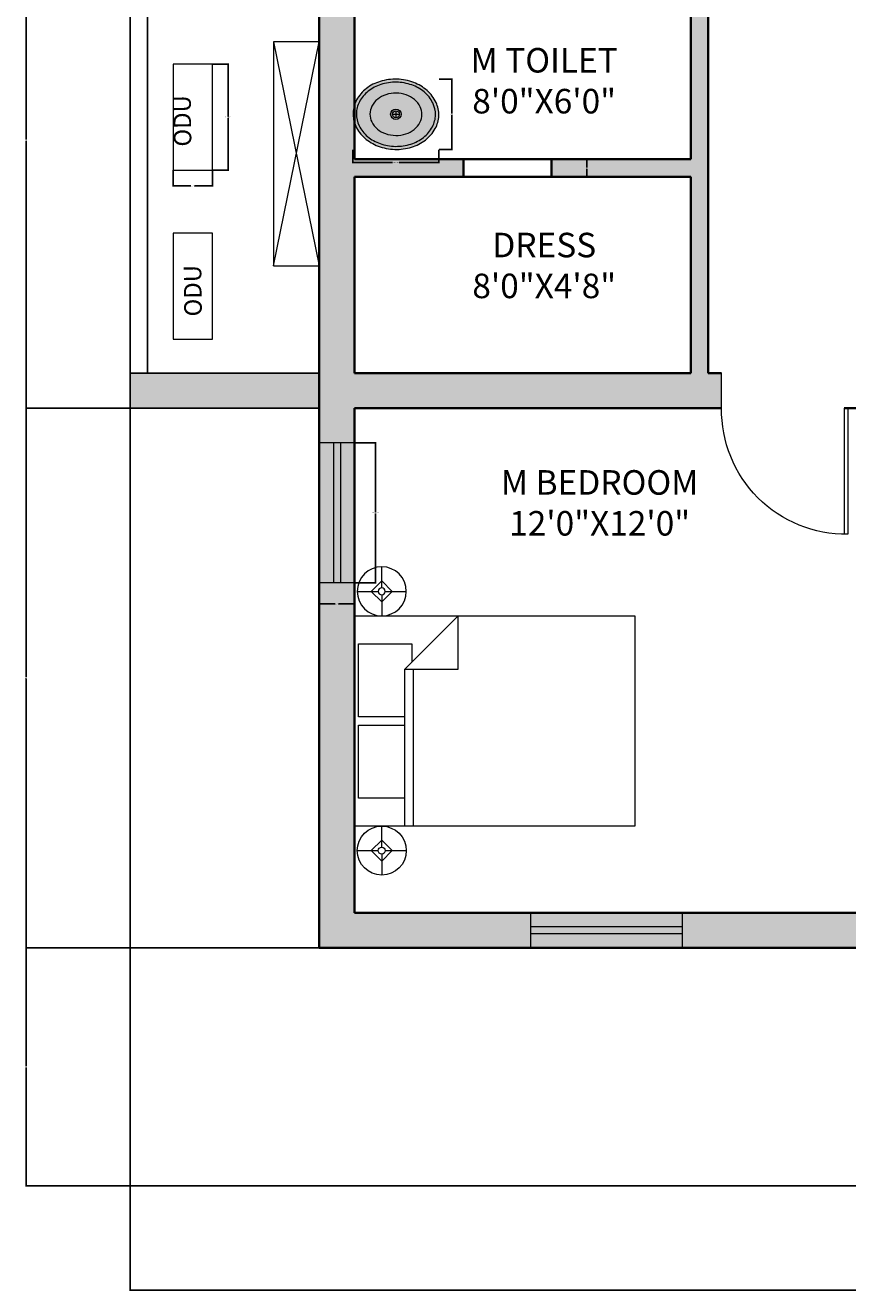
# Model space of a CAD drawing. Units: inches. Extents: x -382 to 250, y 518 to 1732.
# Tile 1 of 8: x -382 to -147, y 518 to 879. Entities that reach past the tile are written whole.
import ezdxf

# ---------------------------------------------------------------- set-up
doc = ezdxf.new("R2010")
doc.units = ezdxf.units.IN
doc.header["$MEASUREMENT"] = 0
for name, color, linetype, lineweight in [('A-ANNO-DIMS', 2, 'Continuous', 18), ('A-AREA-IDEN', 7, 'Continuous', 18), ('A-DOOR', 3, 'Continuous', 18), ('A-FLOR-EDGE', 7, 'Continuous', 25), ('A-FLOR-FIXT', 8, 'Continuous', 18), ('A-FLOR-SHFT', 8, 'Continuous', 18), ('A-FURN', 8, 'Continuous', 18), ('A-GLAZ', 4, 'Continuous', 18), ('A-WALL', 7, 'Continuous', 35), ('M-ANNO-TEXT', 7, 'Continuous', 13), ('M-HVAC-EQPM', 4, 'Continuous', 18)]:
    doc.layers.add(name, color=color, linetype=linetype, lineweight=lineweight)
doc.layers.add('A-GLAZ-PATT', color=143, linetype='Continuous', lineweight=13, true_color=0x7aafdf)
doc.layers.add('A-WALL-PATT', color=251, linetype='Continuous', lineweight=13, true_color=0x636466)
doc.styles.get("Standard").update_dxf_attribs({"font": 'arial.ttf'})
doc.dimstyles.get("Standard").update_dxf_attribs({"dimtxt": 0.18, "dimasz": 0.18, "dimexe": 0.18, "dimexo": 0.0625, "dimgap": 0.09, "dimtad": 0, "dimtih": 1, "dimtoh": 1, "dimdec": 4, "dimzin": 0, "dimdsep": 46, "dimtxsty": 'Standard', "dimcen": 0.09, "dimadec": 0, "dimazin": 0, "dimtfac": 1, "dimtdec": 4, "dimtofl": 0, "dimtmove": 0, "dimatfit": 3, "dimfxl": 1, "dimtolj": 1, "dimtzin": 0, "dimarcsym": 0})

# ---------------------------------------------------------------- blocks, each defined once
blk = doc.blocks.new('Bed - Queen')
for p, q in [((0, -80.00003), (0, 0)), ((0, 0), (59.99999, 0)), ((59.99999, 0), (59.99999, -80.00003)), ((7.99999, -1.2), (28.79998, -1.2)), ((7.99999, -14.4), (7.99999, -1.2)), ((28.79998, -1.2), (28.79998, -14.4)), ((31.19999, -1.2), (51.99999, -1.2)), ((31.19999, -14.4), (31.19999, -1.2)), ((51.99999, -1.2), (51.99999, -16.4)), ((0, -14.4), (44.8, -14.4)), ((59.99999, -29.6), (44.8, -14.4)), ((44.8, -14.4), (44.8, -29.6)), ((44.8, -16.8), (0, -16.8)), ((51.99999, -16.4), (46.79936, -16.4)), ((44.8, -29.6), (59.99999, -29.6)), ((59.99999, -80.00003), (0, -80.00003))]:
    blk.add_line(p, q)
blk = doc.blocks.new('Lamp - Table')
for p, q in [((0, 7), (0, 1)), ((-1, 0), (-7, 0)), ((0, 3), (-3, 0)), ((-3, 0), (0, -3)), ((3, 0), (0, 3)), ((0, -3), (3, 0)), ((1, 0), (7, 0)), ((0, -1), (0, -7))]:
    blk.add_line(p, q)
for radius in [7, 1]:
    blk.add_circle((0, 0), radius)
blk = doc.blocks.new('Sink - Oval top')
for p, q in [((-1, 0), (1, 0)), ((0, 1), (0, -1))]:
    blk.add_line(p, q)
for points in [[(-12.23, 0.39, 0.117634), (-11.46, -3.36, 0.104469), (-8.88, -6.8, 0.090016), (-5.08, -9.07, 0.08192), (-0.32, -10.02, 0.08192), (4.49, -9.38, 0.090016), (8.42, -7.36, 0.104469), (11.22, -4.09, 0.117634), (12.23, -0.39, 0.117634), (11.46, 3.36, 0.104469), (8.88, 6.8, 0.090016), (5.08, 9.07, 0.08192), (0.32, 10.02, 0.08192), (-4.49, 9.38, 0.090016), (-8.42, 7.36, 0.104469), (-11.22, 4.09, 0.117634)], [(-11.29, 0.16, 0.118622), (-10.52, -3.25, 0.104678), (-8.07, -6.36, 0.089562), (-4.54, -8.37, 0.081185), (-0.13, -9.15, 0.081185), (4.3, -8.49, 0.089562), (7.89, -6.58, 0.104678), (10.42, -3.55, 0.118622), (11.29, -0.16, 0.118622), (10.52, 3.25, 0.104678), (8.07, 6.36, 0.089562), (4.54, 8.37, 0.081185), (0.13, 9.15, 0.081185), (-4.3, 8.49, 0.089562), (-7.89, 6.58, 0.104678), (-10.42, 3.55, 0.118622)], [(-7.42, 0.08, 0.118283), (-6.91, -2.17, 0.104607), (-5.29, -4.21, 0.089718), (-2.97, -5.53, 0.081436), (-0.07, -6.04, 0.081436), (2.84, -5.59, 0.089718), (5.2, -4.33, 0.104607), (6.86, -2.32, 0.118283), (7.42, -0.08, 0.118283), (6.91, 2.17, 0.104607), (5.29, 4.21, 0.089718), (2.97, 5.53, 0.081436), (0.07, 6.04, 0.081436), (-2.84, 5.59, 0.089718), (-5.2, 4.33, 0.104607), (-6.86, 2.32, 0.118283)]]:
    blk.add_lwpolyline(points, format="xyb", close=True)
for radius in [1.5, 1]:
    blk.add_circle((0, 0), radius)
blk = doc.blocks.new('WIN-43_2IN')
for p, q in [((0, 10), (0, 0)), ((43.2, 10), (43.2, 0)), ((0, 6), (43.2, 6)), ((0, 4), (43.2, 4))]:
    blk.add_line(p, q)
blk = doc.blocks.new('WIN-40IN')
for p, q in [((10, 40), (0, 40)), ((4, 40), (4, 0)), ((6, 40), (6, 0)), ((10, 0), (0, 0))]:
    blk.add_line(p, q)
blk = doc.blocks.new('DOOR-SWING-36IN')
for p, q in [((-1, 0), (-1, 36)), ((0, 0), (0, 36))]:
    blk.add_line(p, q)
blk.add_arc((-0.5, 0.5), 35.5, 89.1931, 180.8069)
blk = doc.blocks.new('ODU-SIDE-LEDGE')
blk.add_lwpolyline([(0, 0), (11.15, 0), (11.15, 30.22), (0, 30.22)], close=True)
blk = doc.blocks.new('*D44')
at = {"layer": 'A-ANNO-DIMS', "color": 0, "lineweight": -2, "transparency": 16777216}
for p, q in [((-288.63, 843.79), (-288.63, 839.99)), ((-264.08, 843.79), (-264.08, 839.99)), ((-288.45, 840.17), (-277.29, 840.17)), ((-264.26, 840.17), (-275.42, 840.17))]:
    blk.add_line(p, q, dxfattribs=at)
at = {"layer": 'A-ANNO-DIMS', "color": 0, "transparency": 16777216}
for points in [[(-288.45, 840.2), (-288.45, 840.14), (-288.63, 840.17)], [(-264.26, 840.2), (-264.26, 840.14), (-264.08, 840.17)]]:
    blk.add_solid(points, dxfattribs=at)
at = {"layer": 'Defpoints', "color": 0, "transparency": 16777216}
for p in [(-288.63, 843.86), (-264.08, 843.86), (-264.08, 840.17)]:
    blk.add_point(p, dxfattribs=at)
at = {"layer": 'A-ANNO-DIMS', "color": 0, "transparency": 16777216, "insert": (-276.36, 840.17), "char_height": 0.18, "attachment_point": 5}
blk.add_mtext('\\A1;BASIN 25 TYP.', dxfattribs=at)
blk = doc.blocks.new('*D45')
at = {"layer": 'A-ANNO-DIMS', "color": 0, "lineweight": -2, "transparency": 16777216}
for p, q in [((-264.02, 863.99), (-260.22, 863.99)), ((-260.4, 863.81), (-260.4, 854.11)), ((-260.4, 844.04), (-260.4, 853.74)), ((-264.02, 843.86), (-260.22, 843.86))]:
    blk.add_line(p, q, dxfattribs=at)
at = {"layer": 'A-ANNO-DIMS', "color": 0, "transparency": 16777216}
for points in [[(-260.43, 863.81), (-260.37, 863.81), (-260.4, 863.99)], [(-260.43, 844.04), (-260.37, 844.04), (-260.4, 843.86)]]:
    blk.add_solid(points, dxfattribs=at)
at = {"layer": 'Defpoints', "color": 0, "transparency": 16777216}
for p in [(-264.08, 863.99), (-260.4, 863.99), (-264.08, 843.86)]:
    blk.add_point(p, dxfattribs=at)
at = {"layer": 'A-ANNO-DIMS', "color": 0, "transparency": 16777216, "insert": (-260.4, 853.92), "char_height": 0.18, "attachment_point": 5}
blk.add_mtext('\\A1;20 TYP.', dxfattribs=at)
blk = doc.blocks.new('*D56')
at = {"layer": 'A-ANNO-DIMS', "color": 0, "lineweight": -2, "transparency": 16777216}
for p, q in [((-328.68, 868.24), (-324.03, 868.24)), ((-324.21, 868.06), (-324.21, 853.31)), ((-324.21, 838.19), (-324.21, 852.94)), ((-328.68, 838.01), (-324.03, 838.01))]:
    blk.add_line(p, q, dxfattribs=at)
at = {"layer": 'A-ANNO-DIMS', "color": 0, "transparency": 16777216}
for points in [[(-324.24, 868.06), (-324.18, 868.06), (-324.21, 868.24)], [(-324.24, 838.19), (-324.18, 838.19), (-324.21, 838.01)]]:
    blk.add_solid(points, dxfattribs=at)
at = {"layer": 'Defpoints', "color": 0, "transparency": 16777216}
for p in [(-328.74, 868.24), (-324.21, 868.24), (-328.74, 838.01)]:
    blk.add_point(p, dxfattribs=at)
at = {"layer": 'A-ANNO-DIMS', "color": 0, "transparency": 16777216, "insert": (-324.21, 853.13), "char_height": 0.18, "attachment_point": 5}
blk.add_mtext('\\A1;SIDE ODU 30 TYP.', dxfattribs=at)
blk = doc.blocks.new('*D57')
at = {"layer": 'A-ANNO-DIMS', "color": 0, "lineweight": -2, "transparency": 16777216}
for p, q in [((-339.89, 837.95), (-339.89, 833.3)), ((-328.74, 837.95), (-328.74, 833.3)), ((-339.71, 833.48), (-334.84, 833.48)), ((-328.92, 833.48), (-333.8, 833.48))]:
    blk.add_line(p, q, dxfattribs=at)
at = {"layer": 'A-ANNO-DIMS', "color": 0, "transparency": 16777216}
for points in [[(-339.71, 833.51), (-339.71, 833.45), (-339.89, 833.48)], [(-328.92, 833.51), (-328.92, 833.45), (-328.74, 833.48)]]:
    blk.add_solid(points, dxfattribs=at)
at = {"layer": 'Defpoints', "color": 0, "transparency": 16777216}
for p in [(-339.89, 838.01), (-328.74, 838.01), (-328.74, 833.48)]:
    blk.add_point(p, dxfattribs=at)
at = {"layer": 'A-ANNO-DIMS', "color": 0, "transparency": 16777216, "insert": (-334.32, 833.48), "char_height": 0.18, "attachment_point": 5}
blk.add_mtext('\\A1;11 TYP.', dxfattribs=at)
blk = doc.blocks.new('*D70')
at = {"layer": 'A-ANNO-DIMS', "color": 0, "lineweight": -2, "transparency": 16777216}
for p, q in [((-288.15, 760.19), (-282.04, 760.19)), ((-282.22, 760.01), (-282.22, 740.38)), ((-282.22, 720.37), (-282.22, 740.01)), ((-288.15, 720.19), (-282.04, 720.19))]:
    blk.add_line(p, q, dxfattribs=at)
at = {"layer": 'A-ANNO-DIMS', "color": 0, "transparency": 16777216}
for points in [[(-282.25, 760.01), (-282.19, 760.01), (-282.22, 760.19)], [(-282.25, 720.37), (-282.19, 720.37), (-282.22, 720.19)]]:
    blk.add_solid(points, dxfattribs=at)
at = {"layer": 'Defpoints', "color": 0, "transparency": 16777216}
for p in [(-288.22, 760.19), (-282.22, 760.19), (-288.22, 720.19)]:
    blk.add_point(p, dxfattribs=at)
at = {"layer": 'A-ANNO-DIMS', "color": 0, "transparency": 16777216, "insert": (-282.22, 740.19), "char_height": 0.18, "attachment_point": 5}
blk.add_mtext('\\A1;WINDOW B 40 TYP.', dxfattribs=at)
blk = doc.blocks.new('*D71')
at = {"layer": 'A-ANNO-DIMS', "color": 0, "lineweight": -2, "transparency": 16777216}
for p, q in [((-298.22, 720.13), (-298.22, 714.01)), ((-288.22, 720.13), (-288.22, 714.01)), ((-298.04, 714.19), (-293.73, 714.19)), ((-288.4, 714.19), (-292.7, 714.19))]:
    blk.add_line(p, q, dxfattribs=at)
at = {"layer": 'A-ANNO-DIMS', "color": 0, "transparency": 16777216}
for points in [[(-298.04, 714.22), (-298.04, 714.16), (-298.22, 714.19)], [(-288.4, 714.22), (-288.4, 714.16), (-288.22, 714.19)]]:
    blk.add_solid(points, dxfattribs=at)
at = {"layer": 'Defpoints', "color": 0, "transparency": 16777216}
for p in [(-298.22, 720.19), (-288.22, 720.19), (-288.22, 714.19)]:
    blk.add_point(p, dxfattribs=at)
at = {"layer": 'A-ANNO-DIMS', "color": 0, "transparency": 16777216, "insert": (-293.22, 714.19), "char_height": 0.18, "attachment_point": 5}
blk.add_mtext('\\A1;10 TYP.', dxfattribs=at)
blk = doc.blocks.new('*D74')
at = {"layer": 'A-ANNO-DIMS', "color": 0, "lineweight": -2, "transparency": 16777216}
for p, q in [((-352.22, 770.01), (-352.22, 518.19)), ((219.78, 616.01), (219.78, 518.19)), ((-352.04, 518.37), (-66.5, 518.37)), ((219.6, 518.37), (-65.93, 518.37))]:
    blk.add_line(p, q, dxfattribs=at)
at = {"layer": 'A-ANNO-DIMS', "color": 0, "transparency": 16777216}
for points in [[(-352.04, 518.4), (-352.04, 518.34), (-352.22, 518.37)], [(219.6, 518.4), (219.6, 518.34), (219.78, 518.37)]]:
    blk.add_solid(points, dxfattribs=at)
at = {"layer": 'Defpoints', "color": 0, "transparency": 16777216}
for p in [(-352.22, 770.07), (219.78, 616.07), (219.78, 518.37)]:
    blk.add_point(p, dxfattribs=at)
at = {"layer": 'A-ANNO-DIMS', "color": 0, "transparency": 16777216, "insert": (-66.22, 518.37), "char_height": 0.18, "attachment_point": 5}
blk.add_mtext('\\A1;572', dxfattribs=at)
blk = doc.blocks.new('*D79')
at = {"layer": 'A-ANNO-DIMS', "color": 0, "lineweight": -2, "transparency": 16777216}
for p, q in [((-298.28, 770.07), (-382.1, 770.07)), ((-381.92, 769.89), (-381.92, 693.25)), ((-381.92, 616.25), (-381.92, 692.89)), ((-298.28, 616.07), (-382.1, 616.07))]:
    blk.add_line(p, q, dxfattribs=at)
at = {"layer": 'A-ANNO-DIMS', "color": 0, "transparency": 16777216}
for points in [[(-381.95, 769.89), (-381.89, 769.89), (-381.92, 770.07)], [(-381.95, 616.25), (-381.89, 616.25), (-381.92, 616.07)]]:
    blk.add_solid(points, dxfattribs=at)
at = {"layer": 'Defpoints', "color": 0, "transparency": 16777216}
for p in [(-381.92, 770.07), (-298.22, 770.07), (-298.22, 616.07)]:
    blk.add_point(p, dxfattribs=at)
at = {"layer": 'A-ANNO-DIMS', "color": 0, "transparency": 16777216, "insert": (-381.92, 693.07), "char_height": 0.18, "attachment_point": 5}
blk.add_mtext('\\A1;154', dxfattribs=at)
blk = doc.blocks.new('*D80')
at = {"layer": 'A-ANNO-DIMS', "color": 0, "lineweight": -2, "transparency": 16777216}
for p, q in [((-352.28, 923.07), (-382.1, 923.07)), ((-381.92, 922.89), (-381.92, 846.75)), ((-381.92, 770.25), (-381.92, 846.39)), ((-352.28, 770.07), (-382.1, 770.07))]:
    blk.add_line(p, q, dxfattribs=at)
at = {"layer": 'A-ANNO-DIMS', "color": 0, "transparency": 16777216}
for points in [[(-381.95, 922.89), (-381.89, 922.89), (-381.92, 923.07)], [(-381.95, 770.25), (-381.89, 770.25), (-381.92, 770.07)]]:
    blk.add_solid(points, dxfattribs=at)
at = {"layer": 'Defpoints', "color": 0, "transparency": 16777216}
for p in [(-381.92, 923.07), (-352.22, 923.07), (-352.22, 770.07)]:
    blk.add_point(p, dxfattribs=at)
at = {"layer": 'A-ANNO-DIMS', "color": 0, "transparency": 16777216, "insert": (-381.92, 846.57), "char_height": 0.18, "attachment_point": 5}
blk.add_mtext('\\A1;153', dxfattribs=at)
blk = doc.blocks.new('*D82')
at = {"layer": 'A-ANNO-DIMS', "color": 0, "lineweight": -2, "transparency": 16777216}
for p, q in [((-298.28, 616.07), (-382.1, 616.07)), ((-381.92, 615.89), (-381.92, 582.25)), ((-381.92, 548.25), (-381.92, 581.89)), ((38.72, 548.07), (-382.1, 548.07))]:
    blk.add_line(p, q, dxfattribs=at)
at = {"layer": 'A-ANNO-DIMS', "color": 0, "transparency": 16777216}
for points in [[(-381.95, 615.89), (-381.89, 615.89), (-381.92, 616.07)], [(-381.95, 548.25), (-381.89, 548.25), (-381.92, 548.07)]]:
    blk.add_solid(points, dxfattribs=at)
at = {"layer": 'Defpoints', "color": 0, "transparency": 16777216}
for p in [(-381.92, 616.07), (-298.22, 616.07), (38.78, 548.07)]:
    blk.add_point(p, dxfattribs=at)
at = {"layer": 'A-ANNO-DIMS', "color": 0, "transparency": 16777216, "insert": (-381.92, 582.07), "char_height": 0.18, "attachment_point": 5}
blk.add_mtext('\\A1;68', dxfattribs=at)
blk = doc.blocks.new('*D85')
at = {"layer": 'A-ANNO-DIMS', "color": 0, "lineweight": -2, "transparency": 16777216}
for p, q in [((-192.28, 841.07), (-222.1, 841.07)), ((-221.92, 840.89), (-221.92, 838.75)), ((-221.92, 836.25), (-221.92, 838.39)), ((-192.28, 836.07), (-222.1, 836.07))]:
    blk.add_line(p, q, dxfattribs=at)
at = {"layer": 'A-ANNO-DIMS', "color": 0, "transparency": 16777216}
for points in [[(-221.95, 840.89), (-221.89, 840.89), (-221.92, 841.07)], [(-221.95, 836.25), (-221.89, 836.25), (-221.92, 836.07)]]:
    blk.add_solid(points, dxfattribs=at)
at = {"layer": 'Defpoints', "color": 0, "transparency": 16777216}
for p in [(-221.92, 841.07), (-192.22, 841.07), (-192.22, 836.07)]:
    blk.add_point(p, dxfattribs=at)
at = {"layer": 'A-ANNO-DIMS', "color": 0, "transparency": 16777216, "insert": (-221.92, 838.57), "char_height": 0.18, "attachment_point": 5}
blk.add_mtext('\\A1;5', dxfattribs=at)

msp = doc.modelspace()

# ---------------------------------------------------------------- hatches: boundary and pattern name
at = {"layer": 'A-GLAZ-PATT'}
h = msp.add_hatch(color=256, dxfattribs=at)
h.dxf.hatch_style = 1
h.paths.add_polyline_path([(-294.215, 760.1943), (-298.215, 760.1943), (-298.215, 720.1943), (-294.215, 720.1943)])
h = msp.add_hatch(color=256, dxfattribs=at)
h.dxf.hatch_style = 1
h.paths.add_polyline_path([(-292.215, 760.1943), (-294.215, 760.1943), (-294.215, 720.1943), (-292.215, 720.1943)])
h = msp.add_hatch(color=256, dxfattribs=at)
h.dxf.hatch_style = 1
h.paths.add_polyline_path([(-288.215, 760.1943), (-292.215, 760.1943), (-292.215, 720.1943), (-288.215, 720.1943)])
h = msp.add_hatch(color=256, dxfattribs=at)
h.dxf.hatch_style = 1
h.paths.add_polyline_path([(-194.615, 626.0687), (-237.815, 626.0687), (-237.815, 622.0687), (-194.615, 622.0687)])
h = msp.add_hatch(color=256, dxfattribs=at)
h.dxf.hatch_style = 1
h.paths.add_polyline_path([(-194.615, 622.0687), (-237.815, 622.0687), (-237.815, 620.0687), (-194.615, 620.0687)])
h = msp.add_hatch(color=256, dxfattribs=at)
h.dxf.hatch_style = 1
h.paths.add_polyline_path([(-194.615, 620.0687), (-237.815, 620.0687), (-237.815, 616.0687), (-194.615, 616.0687)])
at = {"layer": 'A-WALL-PATT'}
h = msp.add_hatch(color=256, dxfattribs=at)
h.dxf.hatch_style = 1
h.paths.add_polyline_path([(-298.215, 913.0687), (-298.215, 906.5114), (-292.215, 906.5114), (-292.215, 882.5114), (-298.215, 882.5114), (-298.215, 836.0687), (-298.215, 810.633), (-298.215, 770.0687), (-298.215, 760.1943), (-288.215, 760.1943), (-288.215, 770.0687), (-183.4355, 770.0687), (-183.4355, 780.0687), (-187.215, 780.0687), (-187.215, 836.0687), (-187.215, 913.0687), (-182.7819, 913.0687), (-182.7819, 923.0687), (-288.215, 923.0687), (-288.215, 935.4246), (-298.215, 935.4246)])
h.paths.add_polyline_path([(-288.215, 913.0687), (-192.215, 913.0687), (-192.215, 841.0687), (-231.9873, 841.0687), (-231.9873, 836.0687), (-192.215, 836.0687), (-192.215, 780.0687), (-288.215, 780.0687), (-288.215, 836.0687), (-257.0354, 836.0687), (-257.0354, 841.0687), (-288.215, 841.0687), (-288.215, 851.5748, -0.08437411), (-288.5907, 854.3175, -0.06817478), (-288.215, 856.5282)], flags=16)
h.paths.add_polyline_path([(-251.7597, 913.0687), (-230.7597, 913.0687), (-230.7597, 905.0687), (-237.2597, 905.0687), (-235.2598, 899.0688, -0.50132349), (-240.215, 880.2076, -0.13289091), (-242.3044, 880.2076, -0.50131678), (-247.2598, 899.0686), (-245.2597, 905.0687), (-248.2597, 905.0687), (-248.2597, 903.5687), (-251.2597, 903.5687), (-251.2597, 905.0687), (-251.7597, 905.0687)], flags=0)
h.paths.add_polyline_path([(-250.0097, 912.0687), (-232.7597, 912.0687, -0.41421356), (-231.7597, 911.3187), (-231.7597, 907.0687, -0.41421356), (-232.5097, 906.0687), (-249.7597, 906.0687, -0.41421356), (-250.7597, 906.8187), (-250.7597, 911.0687, -0.41421356)], flags=0)
h.paths.add_polyline_path([(-280.8452, 863.304, -0.08191995), (-276.0343, 863.9392, -0.08191995), (-271.2743, 862.9956, -0.09001579), (-267.4783, 860.7269, -0.10446928), (-264.8925, 857.2852, -0.11763426), (-264.1233, 853.5291, -0.11763426), (-265.1327, 849.8303, -0.10446928), (-267.9347, 846.5623, -0.09001579), (-271.8689, 844.5426, -0.08191995), (-276.6798, 843.9075, -0.08191995), (-281.4398, 844.851, -0.09001579), (-285.2358, 847.1198, -0.10446928), (-287.8216, 850.5614, -0.11763426), (-288.5907, 854.3175, -0.11763426), (-287.5814, 858.0163, -0.10446928), (-284.7794, 861.2843, -0.09001579)], flags=16)
h.paths.add_polyline_path([(-280.6571, 862.4148, -0.0811847), (-276.2281, 863.0748, -0.0811847), (-271.8193, 862.2903, -0.08956207), (-268.2852, 860.2819, -0.10467817), (-265.8411, 857.1765, -0.1186217), (-265.0707, 853.7642, -0.1186217), (-265.937, 850.3751, -0.10467817), (-268.4676, 847.3397, -0.08956207), (-272.0569, 845.4318, -0.0811847), (-276.486, 844.7718, -0.0811847), (-280.8947, 845.5563, -0.08956207), (-284.4288, 847.5647, -0.10467817), (-286.8729, 850.6701, -0.1186217), (-287.6433, 854.0824, -0.1186217), (-286.7771, 857.4715, -0.10467817), (-284.2464, 860.5069, -0.08956207)], flags=0)
h.paths.add_polyline_path([(-279.1993, 859.5164, -0.08143608), (-276.2895, 859.9601, -0.08143608), (-273.3904, 859.4514, -0.08971796), (-271.0622, 858.1333, -0.10460746), (-269.45, 856.0908, -0.11828257), (-268.9366, 853.8403, -0.11828257), (-269.5002, 851.6019, -0.10460746), (-271.1577, 849.596, -0.08971796), (-273.5148, 848.3302, -0.08143608), (-276.4245, 847.8865, -0.08143608), (-279.3236, 848.3952, -0.08971796), (-281.6518, 849.7133, -0.10460746), (-283.2641, 851.7558, -0.11828257), (-283.7775, 854.0063, -0.11828257), (-283.2139, 856.2447, -0.10460746), (-281.5563, 858.2507, -0.08971796)], flags=0)
h = msp.add_hatch(color=256, dxfattribs=at)
h.dxf.hatch_style = 1
h.paths.add_polyline_path([(-298.215, 780.0687), (-352.215, 780.0687), (-352.215, 770.0687), (-298.215, 770.0687)])
h = msp.add_hatch(color=256, dxfattribs=at)
h.dxf.hatch_style = 1
h.paths.add_polyline_path([(-288.215, 720.1943), (-298.215, 720.1943), (-298.215, 616.0687), (-237.815, 616.0687), (-237.815, 626.0687), (-288.215, 626.0687)])
h = msp.add_hatch(color=256, dxfattribs=at)
h.dxf.hatch_style = 1
h.paths.add_polyline_path([(-144.215, 626.0687), (-194.615, 626.0687), (-194.615, 616.0687), (-144.215, 616.0687)])

# ---------------------------------------------------------------- linework, layer by layer
at = {"layer": 'A-DOOR'}
msp.add_line((-183.4355, 770.0687), (-183.4355, 780.0687), dxfattribs=at)
at = {"layer": 'A-FLOR-EDGE'}
for p, q in [((-352.215, 770.0687), (-352.215, 923.0687)), ((-347.215, 780.0687), (-347.215, 913.0687)), ((-298.215, 780.0687), (-352.215, 780.0687)), ((-298.215, 770.0687), (-352.215, 770.0687))]:
    msp.add_line(p, q, dxfattribs=at)
at = {"layer": 'A-FLOR-SHFT'}
for p, q in [((-311.3169, 810.633), (-298.215, 874.5687)), ((-311.3169, 874.5687), (-298.215, 810.633))]:
    msp.add_line(p, q, dxfattribs=at)
msp.add_lwpolyline([(-298.215, 874.5687), (-311.3169, 874.5687), (-311.3169, 810.633), (-298.215, 810.633)], close=True, dxfattribs=at)
at = {"layer": 'A-WALL'}
for p, q in [((-298.215, 913.0687), (-298.215, 836.0687)), ((-288.215, 913.0687), (-288.215, 841.0687)), ((-192.215, 913.0687), (-192.215, 841.0687)), ((-187.215, 913.0687), (-187.215, 836.0687)), ((-288.215, 841.0687), (-192.215, 841.0687)), ((-257.0354, 841.0687), (-257.0354, 836.0687)), ((-231.9873, 841.0687), (-231.9873, 836.0687)), ((-298.215, 836.0687), (-298.215, 770.0687)), ((-288.215, 836.0687), (-192.215, 836.0687)), ((-288.215, 836.0687), (-288.215, 780.0687)), ((-192.215, 836.0687), (-192.215, 780.0687)), ((-187.215, 836.0687), (-187.215, 780.0687)), ((-288.215, 780.0687), (-192.215, 780.0687)), ((-187.215, 780.0687), (-183.4355, 780.0687)), ((-298.215, 770.0687), (-298.215, 616.0687)), ((-288.215, 770.0687), (-183.4355, 770.0687)), ((-288.215, 770.0687), (-288.215, 626.0687)), ((-148.4355, 770.0687), (-144.215, 770.0687)), ((-288.215, 626.0687), (-144.215, 626.0687)), ((-298.215, 616.0687), (-144.215, 616.0687))]:
    msp.add_line(p, q, dxfattribs=at)

# ---------------------------------------------------------------- block references
at = {"layer": 'A-DOOR', "extrusion": (0, 0, -1), "zscale": -1, "rotation": 180}
msp.add_blockref('DOOR-SWING-36IN', (147.4355, 770.0687), dxfattribs=at)
at = {"layer": 'A-FLOR-FIXT'}
msp.add_blockref('Sink - Oval top', (-276.357, 853.9233), dxfattribs=at)
at = {"layer": 'A-FURN', "xscale": -1, "rotation": 90}
msp.add_blockref('Lamp - Table', (-280.4036, 717.7765), dxfattribs=at)
at = {"layer": 'A-FURN', "rotation": 90}
for name, p in [('Bed - Queen', (-288.215, 650.7765)), ('Lamp - Table', (-280.4036, 643.7765))]:
    msp.add_blockref(name, p, dxfattribs=at)
at = {"layer": 'A-GLAZ'}
msp.add_blockref('WIN-40IN', (-298.215, 720.194), dxfattribs=at)
at = {"layer": 'A-GLAZ', "rotation": 180}
msp.add_blockref('WIN-43_2IN', (-194.6151, 626.0684), dxfattribs=at)
at = {"layer": 'M-HVAC-EQPM'}
for p in [(-339.89, 838.0139), (-339.89, 789.764)]:
    msp.add_blockref('ODU-SIDE-LEDGE', p, dxfattribs=at)

# ---------------------------------------------------------------- texts
at = {"layer": 'A-AREA-IDEN', "char_height": 7, "attachment_point": 1}
for s, insert in [('\\pxqc;M TOILET\\P8\'0"X6\'0"', (-273.8832, 872.8345)), ('\\pxqc;DRESS\\P8\'0"X4\'8"', (-273.8587, 820.1102)), ('\\pxqc;M BEDROOM \\P12\'0"X12\'0"', (-258.047, 752.359))]:
    msp.add_mtext_dynamic_manual_height_columns(s, width=79.656175, gutter_width=1, heights=[0], dxfattribs=dict(at, insert=insert))
at = {"layer": 'M-ANNO-TEXT', "char_height": 5, "attachment_point": 1, "rotation": 90.712646}
for insert in [(-339.7202, 844.672), (-336.7357, 796.1898)]:
    msp.add_mtext_dynamic_manual_height_columns('ODU', width=13.648337, gutter_width=1, heights=[0], dxfattribs=dict(at, insert=insert))

# ---------------------------------------------------------------- dimensions: what is measured, and where the dimension line sits
at = {"layer": 'A-ANNO-DIMS'}
for base, p1, p2, picture, middle in [((-381.915, 923.0687), (-352.215, 770.0687), (-352.215, 923.0687), '*D80', (-381.915, 846.5687)), ((-221.915, 841.0687), (-192.215, 836.0687), (-192.215, 841.0687), '*D85', (-221.915, 838.5687)), ((-381.915, 770.0687), (-298.215, 616.0687), (-298.215, 770.0687), '*D79', (-381.915, 693.0687)), ((-381.915, 616.0687), (38.785, 548.0687), (-298.215, 616.0687), '*D82', (-381.915, 582.0687))]:
    dim = msp.add_linear_dim(base=base, p1=p1, p2=p2, angle=90, dimstyle='Standard', override={"dimdec": 0, "dimlfac": 1, "dimrnd": 0, "dimzin": 0, "dimdsep": 46, "dimlunit": 2}, dxfattribs=at)
    dim.commit()
    dim.dimension.update_dxf_attribs({"geometry": picture, "text_midpoint": middle})
for base, p1, p2, text, picture, middle in [((-324.2088, 868.2368), (-328.7421, 838.0144), (-328.7421, 868.2368), 'SIDE ODU <> TYP.', '*D56', (-324.2088, 853.1256)), ((-260.3989, 863.9916), (-264.0816, 843.855), (-264.0816, 863.9916), '<> TYP.', '*D45', (-260.3989, 853.9233)), ((-282.215, 760.1943), (-288.215, 720.1943), (-288.215, 760.1943), 'WINDOW B <> TYP.', '*D70', (-282.215, 740.1943))]:
    dim = msp.add_linear_dim(base=base, p1=p1, p2=p2, angle=90, text=text, dimstyle='Standard', override={"dimdec": 0, "dimlfac": 1, "dimrnd": 0, "dimzin": 0, "dimdsep": 46, "dimlunit": 2}, dxfattribs=at)
    dim.commit()
    dim.dimension.update_dxf_attribs({"geometry": picture, "text_midpoint": middle})
for base, p1, p2, text, picture, middle in [((-264.0816, 840.1724), (-288.6325, 843.855), (-264.0816, 843.855), 'BASIN <> TYP.', '*D44', (-276.357, 840.1724)), ((-328.7421, 833.481), (-339.89, 838.0144), (-328.7421, 838.0144), '<> TYP.', '*D57', (-334.3161, 833.481)), ((-288.215, 714.1943), (-298.215, 720.1943), (-288.215, 720.1943), '<> TYP.', '*D71', (-293.215, 714.1943))]:
    dim = msp.add_linear_dim(base=base, p1=p1, p2=p2, text=text, dimstyle='Standard', override={"dimdec": 0, "dimlfac": 1, "dimrnd": 0, "dimzin": 0, "dimdsep": 46, "dimlunit": 2}, dxfattribs=at)
    dim.commit()
    dim.dimension.update_dxf_attribs({"geometry": picture, "text_midpoint": middle})
dim = msp.add_linear_dim(base=(219.785, 518.3687), p1=(-352.215, 770.0687), p2=(219.785, 616.0687), dimstyle='Standard', override={"dimdec": 0, "dimlfac": 1, "dimrnd": 0, "dimzin": 0, "dimdsep": 46, "dimlunit": 2}, dxfattribs=at)
dim.commit()
dim.dimension.update_dxf_attribs({"geometry": '*D74', "text_midpoint": (-66.215, 518.3687)})

doc.saveas('drawing.dxf')
